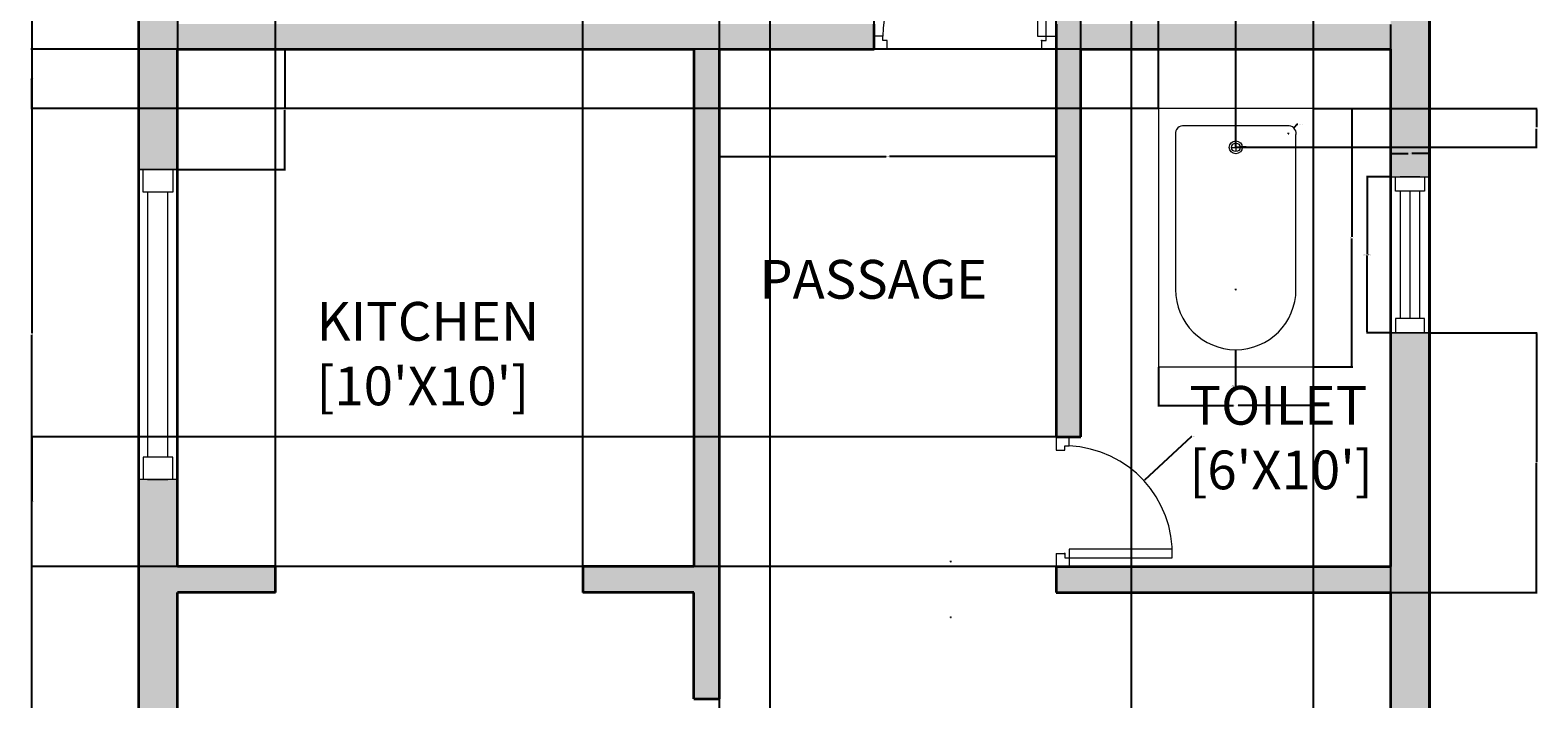
# Model space of a CAD drawing. Units: inches. Extents: x 2203 to 2554, y 381 to 929.
# Tile 2 of 3: x 2203 to 2554, y 570 to 726. Entities that reach past the tile are written whole.
import ezdxf

# ---------------------------------------------------------------- set-up
doc = ezdxf.new("R2010")
doc.units = ezdxf.units.IN
for name, color, linetype, lineweight in [('A-ANNO-DIMS', 2, 'Continuous', 18), ('A-AREA-IDEN', 7, 'Continuous', 18), ('A-DOOR', 239, 'Continuous', 18), ('A-FLOR-FIXT', 8, 'Continuous', 18), ('A-GLAZ', 4, 'Continuous', 18), ('A-WALL', 7, 'Continuous', 35), ('A-WALL-PATT', 250, 'Continuous', 13)]:
    doc.layers.add(name, color=color, linetype=linetype, lineweight=lineweight)
doc.styles.get("Standard").update_dxf_attribs({"font": 'arial.ttf'})
doc.dimstyles.get("Standard").update_dxf_attribs({"dimtxt": 0.18, "dimasz": 0.18, "dimexe": 0.18, "dimexo": 0.0625, "dimgap": 0.09, "dimtad": 0, "dimtih": 1, "dimtoh": 1, "dimdec": 4, "dimzin": 0, "dimdsep": 46, "dimtxsty": 'Standard', "dimcen": 0.09, "dimadec": 0, "dimazin": 0, "dimtfac": 1, "dimtdec": 4, "dimtofl": 0, "dimtmove": 0, "dimatfit": 3, "dimfxl": 1, "dimtolj": 1, "dimtzin": 0, "dimarcsym": 0})

# ---------------------------------------------------------------- blocks, each defined once
blk = doc.blocks.new('WIN-36')
for p, q in [((0, 36.19), (9, 36.19)), ((0, 0), (0, 36.19)), ((0, 36.19), (4.5, 36.19)), ((1.12, 32.87), (1.12, 36.19)), ((6.76, 36.19), (2.25, 36.19)), ((7.88, 36.19), (7.88, 32.87)), ((9, 36.19), (9, 0)), ((7.88, 32.87), (1.12, 32.87)), ((2.25, 32.87), (2.25, 3.32)), ((4.5, 32.87), (4.5, 3.32)), ((6.76, 3.32), (6.76, 32.87)), ((9, 0), (0, 0)), ((2.25, 0), (0, 0)), ((0, 0), (6.76, 0)), ((7.88, 3.32), (1.12, 3.32)), ((1.12, 3.32), (1.12, 0)), ((4.5, 0), (6.76, 0)), ((6.76, 0), (9, 0)), ((7.88, 0), (7.88, 3.32))]:
    blk.add_line(p, q)
blk = doc.blocks.new('WIN-72')
for p, q in [((0, 0), (0, 9)), ((0, 9), (72, 9)), ((5.2, 7.99), (0, 7.99)), ((5.2, 1.13), (5.2, 7.99)), ((66.8, 1.13), (66.8, 7.99)), ((66.8, 7.99), (72, 7.99)), ((72, 9), (72, 0)), ((72, 6.99), (72, 9)), ((0, 6.99), (0, 2.25)), ((0, 0), (0, 4.5)), ((66.8, 6.99), (5.2, 6.99)), ((72, 4.5), (72, 6.99)), ((72, 2.25), (72, 6.99)), ((0, 1.13), (5.2, 1.13)), ((72, 0), (0, 0)), ((5.2, 2.25), (66.8, 2.25)), ((72, 1.13), (66.8, 1.13)), ((72, 0), (72, 2.25))]:
    blk.add_line(p, q)
blk = doc.blocks.new('TUB-36X60')
for p, q in [((17, 51), (19, 51)), ((18, 52), (18, 50))]:
    blk.add_line(p, q)
blk.add_lwpolyline([(36, 60), (0, 60), (0, 0), (36, 0)], close=True)
for points in [[(4, 54), (4, 18)], [(30, 56), (6, 56)], [(32, 18), (32, 54)]]:
    blk.add_lwpolyline(points)
for radius in [1.5, 1]:
    blk.add_circle((18, 51), radius)
for centre, radius, start, end in [((5.75, 54.25), 1.77, 81.8699, 188.1301), ((30.25, 54.25), 1.77, 351.8699, 98.1301), ((18, 18), 14, 180, 0)]:
    blk.add_arc(centre, radius, start, end)
blk = doc.blocks.new('*D17')
at = {"layer": 'A-ANNO-DIMS', "color": 0, "lineweight": -2, "transparency": 16777216}
for p, q in [((2519.54, 691.56), (2513.99, 691.56)), ((2514.17, 691.38), (2514.17, 673.65)), ((2514.17, 655.55), (2514.17, 673.28)), ((2519.54, 655.37), (2513.99, 655.37))]:
    blk.add_line(p, q, dxfattribs=at)
at = {"layer": 'A-ANNO-DIMS', "color": 0, "transparency": 16777216}
for points in [[(2514.14, 691.38), (2514.2, 691.38), (2514.17, 691.56)], [(2514.14, 655.55), (2514.2, 655.55), (2514.17, 655.37)]]:
    blk.add_solid(points, dxfattribs=at)
at = {"layer": 'Defpoints', "color": 0, "transparency": 16777216}
for p in [(2514.17, 691.56), (2519.6, 691.56), (2519.6, 655.37)]:
    blk.add_point(p, dxfattribs=at)
at = {"layer": 'A-ANNO-DIMS', "color": 0, "transparency": 16777216, "insert": (2514.17, 673.46), "char_height": 0.18, "attachment_point": 5}
blk.add_mtext('\\A1;WINDOW 36 TYP.', dxfattribs=at)
blk = doc.blocks.new('*D18')
at = {"layer": 'A-ANNO-DIMS', "color": 0, "lineweight": -2, "transparency": 16777216}
for p, q in [((2519.6, 691.62), (2519.6, 697.17)), ((2519.78, 696.99), (2523.64, 696.99)), ((2528.42, 696.99), (2524.56, 696.99)), ((2528.6, 691.62), (2528.6, 697.17))]:
    blk.add_line(p, q, dxfattribs=at)
at = {"layer": 'A-ANNO-DIMS', "color": 0, "transparency": 16777216}
for points in [[(2519.78, 697.02), (2519.78, 696.96), (2519.6, 696.99)], [(2528.42, 697.02), (2528.42, 696.96), (2528.6, 696.99)]]:
    blk.add_solid(points, dxfattribs=at)
at = {"layer": 'Defpoints', "color": 0, "transparency": 16777216}
for p in [(2528.6, 696.99), (2519.6, 691.56), (2528.6, 691.56)]:
    blk.add_point(p, dxfattribs=at)
at = {"layer": 'A-ANNO-DIMS', "color": 0, "transparency": 16777216, "insert": (2524.1, 696.99), "char_height": 0.18, "attachment_point": 5}
blk.add_mtext('\\A1;9 TYP.', dxfattribs=at)
blk = doc.blocks.new('*D19')
at = {"layer": 'A-ANNO-DIMS', "color": 0, "lineweight": -2, "transparency": 16777216}
for p, q in [((2501.66, 707.44), (2510.78, 707.44)), ((2510.6, 707.26), (2510.6, 677.62)), ((2510.6, 647.62), (2510.6, 677.25)), ((2501.66, 647.44), (2510.78, 647.44))]:
    blk.add_line(p, q, dxfattribs=at)
at = {"layer": 'A-ANNO-DIMS', "color": 0, "transparency": 16777216}
for points in [[(2510.57, 707.26), (2510.63, 707.26), (2510.6, 707.44)], [(2510.57, 647.62), (2510.63, 647.62), (2510.6, 647.44)]]:
    blk.add_solid(points, dxfattribs=at)
at = {"layer": 'Defpoints', "color": 0, "transparency": 16777216}
for p in [(2501.6, 707.44), (2510.6, 707.44), (2501.6, 647.44)]:
    blk.add_point(p, dxfattribs=at)
at = {"layer": 'A-ANNO-DIMS', "color": 0, "transparency": 16777216, "insert": (2510.6, 677.44), "char_height": 0.18, "attachment_point": 5}
blk.add_mtext('\\A1;TUB 60 TYP.', dxfattribs=at)
blk = doc.blocks.new('*D20')
at = {"layer": 'A-ANNO-DIMS', "color": 0, "lineweight": -2, "transparency": 16777216}
for p, q in [((2465.6, 647.37), (2465.6, 638.26)), ((2501.6, 647.37), (2501.6, 638.26)), ((2465.78, 638.44), (2483.07, 638.44)), ((2501.42, 638.44), (2484.13, 638.44))]:
    blk.add_line(p, q, dxfattribs=at)
at = {"layer": 'A-ANNO-DIMS', "color": 0, "transparency": 16777216}
for points in [[(2465.78, 638.47), (2465.78, 638.41), (2465.6, 638.44)], [(2501.42, 638.47), (2501.42, 638.41), (2501.6, 638.44)]]:
    blk.add_solid(points, dxfattribs=at)
at = {"layer": 'Defpoints', "color": 0, "transparency": 16777216}
for p in [(2465.6, 647.44), (2501.6, 647.44), (2501.6, 638.44)]:
    blk.add_point(p, dxfattribs=at)
at = {"layer": 'A-ANNO-DIMS', "color": 0, "transparency": 16777216, "insert": (2483.6, 638.44), "char_height": 0.18, "attachment_point": 5}
blk.add_mtext('\\A1;36 TYP.', dxfattribs=at)
blk = doc.blocks.new('*D22')
at = {"layer": 'A-ANNO-DIMS', "color": 0, "lineweight": -2, "transparency": 16777216}
for p, q in [((2228.54, 904.06), (2203.5, 904.06)), ((2203.68, 903.88), (2203.68, 655.25)), ((2203.68, 406.24), (2203.68, 654.88)), ((2228.54, 406.06), (2203.5, 406.06))]:
    blk.add_line(p, q, dxfattribs=at)
at = {"layer": 'A-ANNO-DIMS', "color": 0, "transparency": 16777216}
for points in [[(2203.65, 903.88), (2203.71, 903.88), (2203.68, 904.06)], [(2203.65, 406.24), (2203.71, 406.24), (2203.68, 406.06)]]:
    blk.add_solid(points, dxfattribs=at)
at = {"layer": 'Defpoints', "color": 0, "transparency": 16777216}
for p in [(2203.68, 904.06), (2228.6, 904.06), (2228.6, 406.06)]:
    blk.add_point(p, dxfattribs=at)
at = {"layer": 'A-ANNO-DIMS', "color": 0, "transparency": 16777216, "insert": (2203.68, 655.06), "char_height": 0.18, "attachment_point": 5}
blk.add_mtext('\\A1;498', dxfattribs=at)
blk = doc.blocks.new('*D26')
at = {"layer": 'A-ANNO-DIMS', "color": 0, "lineweight": -2, "transparency": 16777216}
for p, q in [((2237.66, 721.24), (2262.7, 721.24)), ((2262.52, 721.06), (2262.52, 707.43)), ((2262.52, 693.44), (2262.52, 707.07)), ((2237.66, 693.26), (2262.7, 693.26))]:
    blk.add_line(p, q, dxfattribs=at)
at = {"layer": 'A-ANNO-DIMS', "color": 0, "transparency": 16777216}
for points in [[(2262.49, 721.06), (2262.55, 721.06), (2262.52, 721.24)], [(2262.49, 693.44), (2262.55, 693.44), (2262.52, 693.26)]]:
    blk.add_solid(points, dxfattribs=at)
at = {"layer": 'Defpoints', "color": 0, "transparency": 16777216}
for p in [(2237.6, 721.24), (2237.6, 693.26), (2262.52, 693.26)]:
    blk.add_point(p, dxfattribs=at)
at = {"layer": 'A-ANNO-DIMS', "color": 0, "transparency": 16777216, "insert": (2262.52, 707.25), "char_height": 0.18, "attachment_point": 5}
blk.add_mtext('\\A1;27.985', dxfattribs=at)
blk = doc.blocks.new('*D27')
at = {"layer": 'A-ANNO-DIMS', "color": 0, "lineweight": -2, "transparency": 16777216}
for p, q in [((2528.66, 655.37), (2553.7, 655.37)), ((2553.52, 655.19), (2553.52, 625.4)), ((2553.52, 595.24), (2553.52, 625.04)), ((2519.66, 595.06), (2553.7, 595.06))]:
    blk.add_line(p, q, dxfattribs=at)
at = {"layer": 'A-ANNO-DIMS', "color": 0, "transparency": 16777216}
for points in [[(2553.49, 655.19), (2553.55, 655.19), (2553.52, 655.37)], [(2553.49, 595.24), (2553.55, 595.24), (2553.52, 595.06)]]:
    blk.add_solid(points, dxfattribs=at)
at = {"layer": 'Defpoints', "color": 0, "transparency": 16777216}
for p in [(2528.6, 655.37), (2553.52, 655.37), (2519.6, 595.06)]:
    blk.add_point(p, dxfattribs=at)
at = {"layer": 'A-ANNO-DIMS', "color": 0, "transparency": 16777216, "insert": (2553.52, 625.22), "char_height": 0.18, "attachment_point": 5}
blk.add_mtext('\\A1;60.31', dxfattribs=at)
blk = doc.blocks.new('*D29')
at = {"layer": 'A-ANNO-DIMS', "color": 0, "lineweight": -2, "transparency": 16777216}
for p, q in [((2363.6, 721.18), (2363.6, 696.14)), ((2441.82, 721.18), (2441.82, 696.14)), ((2363.78, 696.32), (2402.32, 696.32)), ((2441.64, 696.32), (2403.1, 696.32))]:
    blk.add_line(p, q, dxfattribs=at)
at = {"layer": 'A-ANNO-DIMS', "color": 0, "transparency": 16777216}
for points in [[(2363.78, 696.35), (2363.78, 696.29), (2363.6, 696.32)], [(2441.64, 696.35), (2441.64, 696.29), (2441.82, 696.32)]]:
    blk.add_solid(points, dxfattribs=at)
at = {"layer": 'Defpoints', "color": 0, "transparency": 16777216}
for p in [(2363.6, 721.24), (2441.82, 721.24), (2363.6, 696.32)]:
    blk.add_point(p, dxfattribs=at)
at = {"layer": 'A-ANNO-DIMS', "color": 0, "transparency": 16777216, "insert": (2402.71, 696.32), "char_height": 0.18, "attachment_point": 5}
blk.add_mtext('\\A1;78.23', dxfattribs=at)
blk = doc.blocks.new('*D30')
at = {"layer": 'A-ANNO-DIMS', "color": 0, "lineweight": -2, "transparency": 16777216}
for p, q in [((2237.6, 601.13), (2237.6, 929.16)), ((2237.78, 928.98), (2248.57, 928.98)), ((2260.15, 928.98), (2249.36, 928.98)), ((2260.33, 601.13), (2260.33, 929.16))]:
    blk.add_line(p, q, dxfattribs=at)
at = {"layer": 'A-ANNO-DIMS', "color": 0, "transparency": 16777216}
for points in [[(2237.78, 929.01), (2237.78, 928.95), (2237.6, 928.98)], [(2260.15, 929.01), (2260.15, 928.95), (2260.33, 928.98)]]:
    blk.add_solid(points, dxfattribs=at)
at = {"layer": 'Defpoints', "color": 0, "transparency": 16777216}
for p in [(2260.33, 928.98), (2237.6, 601.06), (2260.33, 601.06)]:
    blk.add_point(p, dxfattribs=at)
at = {"layer": 'A-ANNO-DIMS', "color": 0, "transparency": 16777216, "insert": (2248.96, 928.98), "char_height": 0.18, "attachment_point": 5}
blk.add_mtext('\\A1;22.73', dxfattribs=at)
blk = doc.blocks.new('*D31')
at = {"layer": 'A-ANNO-DIMS', "color": 0, "lineweight": -2, "transparency": 16777216}
for p, q in [((2260.33, 601.13), (2260.33, 929.16)), ((2260.51, 928.98), (2295.75, 928.98)), ((2331.64, 928.98), (2296.4, 928.98)), ((2331.82, 601.13), (2331.82, 929.16))]:
    blk.add_line(p, q, dxfattribs=at)
at = {"layer": 'A-ANNO-DIMS', "color": 0, "transparency": 16777216}
for points in [[(2260.51, 929.01), (2260.51, 928.95), (2260.33, 928.98)], [(2331.64, 929.01), (2331.64, 928.95), (2331.82, 928.98)]]:
    blk.add_solid(points, dxfattribs=at)
at = {"layer": 'Defpoints', "color": 0, "transparency": 16777216}
for p in [(2331.82, 928.98), (2260.33, 601.06), (2331.82, 601.06)]:
    blk.add_point(p, dxfattribs=at)
at = {"layer": 'A-ANNO-DIMS', "color": 0, "transparency": 16777216, "insert": (2296.08, 928.98), "char_height": 0.18, "attachment_point": 5}
blk.add_mtext('\\A1;71.5', dxfattribs=at)
blk = doc.blocks.new('*D35')
at = {"layer": 'A-ANNO-DIMS', "color": 0, "lineweight": -2, "transparency": 16777216}
for p, q in [((2399.53, 721.31), (2399.53, 746.34)), ((2399.71, 746.16), (2420.28, 746.16)), ((2441.64, 746.16), (2421.08, 746.16)), ((2441.82, 721.31), (2441.82, 746.34))]:
    blk.add_line(p, q, dxfattribs=at)
at = {"layer": 'A-ANNO-DIMS', "color": 0, "transparency": 16777216}
for points in [[(2399.71, 746.19), (2399.71, 746.13), (2399.53, 746.16)], [(2441.64, 746.19), (2441.64, 746.13), (2441.82, 746.16)]]:
    blk.add_solid(points, dxfattribs=at)
at = {"layer": 'Defpoints', "color": 0, "transparency": 16777216}
for p in [(2441.82, 746.16), (2399.53, 721.24), (2441.82, 721.24)]:
    blk.add_point(p, dxfattribs=at)
at = {"layer": 'A-ANNO-DIMS', "color": 0, "transparency": 16777216, "insert": (2420.68, 746.16), "char_height": 0.18, "attachment_point": 5}
blk.add_mtext('\\A1;42.29', dxfattribs=at)
blk = doc.blocks.new('*D37')
at = {"layer": 'A-ANNO-DIMS', "color": 0, "lineweight": -2, "transparency": 16777216}
for p, q in [((2441.76, 631.17), (2203.5, 631.17)), ((2203.68, 630.99), (2203.68, 616.3)), ((2203.68, 601.24), (2203.68, 615.93)), ((2441.76, 601.06), (2203.5, 601.06))]:
    blk.add_line(p, q, dxfattribs=at)
at = {"layer": 'A-ANNO-DIMS', "color": 0, "transparency": 16777216}
for points in [[(2203.65, 630.99), (2203.71, 630.99), (2203.68, 631.17)], [(2203.65, 601.24), (2203.71, 601.24), (2203.68, 601.06)]]:
    blk.add_solid(points, dxfattribs=at)
at = {"layer": 'Defpoints', "color": 0, "transparency": 16777216}
for p in [(2203.68, 631.17), (2441.82, 631.17), (2441.82, 601.06)]:
    blk.add_point(p, dxfattribs=at)
at = {"layer": 'A-ANNO-DIMS', "color": 0, "transparency": 16777216, "insert": (2203.68, 616.12), "char_height": 0.18, "attachment_point": 5}
blk.add_mtext('\\A1;30.104', dxfattribs=at)
blk = doc.blocks.new('*D41')
at = {"layer": 'A-ANNO-DIMS', "color": 0, "lineweight": -2, "transparency": 16777216}
for p, q in [((2375.37, 509.13), (2375.37, 929.16)), ((2375.55, 928.98), (2417.15, 928.98)), ((2459.19, 928.98), (2417.59, 928.98)), ((2459.37, 509.13), (2459.37, 929.16))]:
    blk.add_line(p, q, dxfattribs=at)
at = {"layer": 'A-ANNO-DIMS', "color": 0, "transparency": 16777216}
for points in [[(2375.55, 929.01), (2375.55, 928.95), (2375.37, 928.98)], [(2459.19, 929.01), (2459.19, 928.95), (2459.37, 928.98)]]:
    blk.add_solid(points, dxfattribs=at)
at = {"layer": 'Defpoints', "color": 0, "transparency": 16777216}
for p in [(2459.37, 928.98), (2375.37, 509.06), (2459.37, 509.06)]:
    blk.add_point(p, dxfattribs=at)
at = {"layer": 'A-ANNO-DIMS', "color": 0, "transparency": 16777216, "insert": (2417.37, 928.98), "char_height": 0.18, "attachment_point": 5}
blk.add_mtext('\\A1;84', dxfattribs=at)
blk = doc.blocks.new('*D43')
at = {"layer": 'A-ANNO-DIMS', "color": 0, "lineweight": -2, "transparency": 16777216}
for p, q in [((2363.6, 500.21), (2363.6, 929.16)), ((2363.78, 928.98), (2369.03, 928.98)), ((2375.19, 928.98), (2369.94, 928.98)), ((2375.37, 509.13), (2375.37, 929.16))]:
    blk.add_line(p, q, dxfattribs=at)
at = {"layer": 'A-ANNO-DIMS', "color": 0, "transparency": 16777216}
for points in [[(2363.78, 929.01), (2363.78, 928.95), (2363.6, 928.98)], [(2375.19, 929.01), (2375.19, 928.95), (2375.37, 928.98)]]:
    blk.add_solid(points, dxfattribs=at)
at = {"layer": 'Defpoints', "color": 0, "transparency": 16777216}
for p in [(2375.37, 928.98), (2375.37, 509.06), (2363.6, 500.15)]:
    blk.add_point(p, dxfattribs=at)
at = {"layer": 'A-ANNO-DIMS', "color": 0, "transparency": 16777216, "insert": (2369.49, 928.98), "char_height": 0.18, "attachment_point": 5}
blk.add_mtext('\\A1;11.775', dxfattribs=at)
blk = doc.blocks.new('*D50')
at = {"layer": 'A-ANNO-DIMS', "color": 0, "lineweight": -2, "transparency": 16777216}
for p, q in [((2465.6, 707.5), (2465.6, 929.16)), ((2465.78, 928.98), (2474.39, 928.98)), ((2483.42, 928.98), (2474.81, 928.98)), ((2483.6, 698.5), (2483.6, 929.16))]:
    blk.add_line(p, q, dxfattribs=at)
at = {"layer": 'A-ANNO-DIMS', "color": 0, "transparency": 16777216}
for points in [[(2465.78, 929.01), (2465.78, 928.95), (2465.6, 928.98)], [(2483.42, 929.01), (2483.42, 928.95), (2483.6, 928.98)]]:
    blk.add_solid(points, dxfattribs=at)
at = {"layer": 'Defpoints', "color": 0, "transparency": 16777216}
for p in [(2483.6, 928.98), (2465.6, 707.44), (2483.6, 698.44)]:
    blk.add_point(p, dxfattribs=at)
at = {"layer": 'A-ANNO-DIMS', "color": 0, "transparency": 16777216, "insert": (2474.6, 928.98), "char_height": 0.18, "attachment_point": 5}
blk.add_mtext('\\A1;18', dxfattribs=at)
blk = doc.blocks.new('*D51')
at = {"layer": 'A-ANNO-DIMS', "color": 0, "lineweight": -2, "transparency": 16777216}
for p, q in [((2501.66, 707.44), (2553.7, 707.44)), ((2553.52, 707.26), (2553.52, 703.12)), ((2553.52, 698.62), (2553.52, 702.75)), ((2483.66, 698.44), (2553.7, 698.44))]:
    blk.add_line(p, q, dxfattribs=at)
at = {"layer": 'A-ANNO-DIMS', "color": 0, "transparency": 16777216}
for points in [[(2553.49, 707.26), (2553.55, 707.26), (2553.52, 707.44)], [(2553.49, 698.62), (2553.55, 698.62), (2553.52, 698.44)]]:
    blk.add_solid(points, dxfattribs=at)
at = {"layer": 'Defpoints', "color": 0, "transparency": 16777216}
for p in [(2501.6, 707.44), (2483.6, 698.44), (2553.52, 698.44)]:
    blk.add_point(p, dxfattribs=at)
at = {"layer": 'A-ANNO-DIMS', "color": 0, "transparency": 16777216, "insert": (2553.52, 702.94), "char_height": 0.18, "attachment_point": 5}
blk.add_mtext('\\A1;9', dxfattribs=at)
blk = doc.blocks.new('*D52')
at = {"layer": 'A-ANNO-DIMS', "color": 0, "lineweight": -2, "transparency": 16777216}
for p, q in [((2447.6, 721.31), (2447.6, 929.16)), ((2447.78, 928.98), (2456.39, 928.98)), ((2465.42, 928.98), (2456.81, 928.98)), ((2465.6, 707.5), (2465.6, 929.16))]:
    blk.add_line(p, q, dxfattribs=at)
at = {"layer": 'A-ANNO-DIMS', "color": 0, "transparency": 16777216}
for points in [[(2447.78, 929.01), (2447.78, 928.95), (2447.6, 928.98)], [(2465.42, 929.01), (2465.42, 928.95), (2465.6, 928.98)]]:
    blk.add_solid(points, dxfattribs=at)
at = {"layer": 'Defpoints', "color": 0, "transparency": 16777216}
for p in [(2447.6, 928.98), (2447.6, 721.24), (2465.6, 707.44)]:
    blk.add_point(p, dxfattribs=at)
at = {"layer": 'A-ANNO-DIMS', "color": 0, "transparency": 16777216, "insert": (2456.6, 928.98), "char_height": 0.18, "attachment_point": 5}
blk.add_mtext('\\A1;18', dxfattribs=at)
blk = doc.blocks.new('*D53')
at = {"layer": 'A-ANNO-DIMS', "color": 0, "lineweight": -2, "transparency": 16777216}
for p, q in [((2447.54, 721.24), (2203.5, 721.24)), ((2203.68, 721.06), (2203.68, 714.52)), ((2203.68, 707.62), (2203.68, 714.16)), ((2465.54, 707.44), (2203.5, 707.44))]:
    blk.add_line(p, q, dxfattribs=at)
at = {"layer": 'A-ANNO-DIMS', "color": 0, "transparency": 16777216}
for points in [[(2203.65, 721.06), (2203.71, 721.06), (2203.68, 721.24)], [(2203.65, 707.62), (2203.71, 707.62), (2203.68, 707.44)]]:
    blk.add_solid(points, dxfattribs=at)
at = {"layer": 'Defpoints', "color": 0, "transparency": 16777216}
for p in [(2203.68, 721.24), (2447.6, 721.24), (2465.6, 707.44)]:
    blk.add_point(p, dxfattribs=at)
at = {"layer": 'A-ANNO-DIMS', "color": 0, "transparency": 16777216, "insert": (2203.68, 714.34), "char_height": 0.18, "attachment_point": 5}
blk.add_mtext('\\A1;13.808', dxfattribs=at)
blk = doc.blocks.new('*D55')
at = {"layer": 'A-ANNO-DIMS', "color": 0, "lineweight": -2, "transparency": 16777216}
for p, q in [((2501.6, 739.61), (2501.6, 380.96)), ((2519.6, 727), (2519.6, 380.96)), ((2501.78, 381.14), (2510.39, 381.14)), ((2519.42, 381.14), (2510.81, 381.14))]:
    blk.add_line(p, q, dxfattribs=at)
at = {"layer": 'A-ANNO-DIMS', "color": 0, "transparency": 16777216}
for points in [[(2501.78, 381.17), (2501.78, 381.11), (2501.6, 381.14)], [(2519.42, 381.17), (2519.42, 381.11), (2519.6, 381.14)]]:
    blk.add_solid(points, dxfattribs=at)
at = {"layer": 'Defpoints', "color": 0, "transparency": 16777216}
for p in [(2501.6, 739.68), (2519.6, 727.06), (2519.6, 381.14)]:
    blk.add_point(p, dxfattribs=at)
at = {"layer": 'A-ANNO-DIMS', "color": 0, "transparency": 16777216, "insert": (2510.6, 381.14), "char_height": 0.18, "attachment_point": 5}
blk.add_mtext('\\A1;18', dxfattribs=at)
blk = doc.blocks.new('*D60')
at = {"layer": 'A-ANNO-DIMS', "color": 0, "lineweight": -2, "transparency": 16777216}
for p, q in [((2417.28, 602.26), (2417.46, 602.26)), ((2417.37, 602.17), (2417.37, 602.35)), ((2417.37, 408.35), (2417.37, 480.88)), ((2417.55, 408.35), (2417.37, 408.35))]:
    blk.add_line(p, q, dxfattribs=at)
at = {"layer": 'A-ANNO-DIMS', "color": 0, "transparency": 16777216}
blk.add_solid([(2417.4, 480.88), (2417.34, 480.88), (2417.37, 481.06)], dxfattribs=at)
at = {"layer": 'Defpoints', "color": 0, "transparency": 16777216}
for p in [(2417.37, 602.26), (2417.37, 481.06)]:
    blk.add_point(p, dxfattribs=at)
at = {"layer": 'A-ANNO-DIMS', "color": 0, "transparency": 16777216, "insert": (2418.03, 408.35), "char_height": 0.18, "attachment_point": 5}
blk.add_mtext('\\A1;R121.2', dxfattribs=at)
blk = doc.blocks.new('*D61')
at = {"layer": 'A-ANNO-DIMS', "color": 0, "lineweight": -2, "transparency": 16777216}
for p, q in [((2417.28, 589.31), (2417.46, 589.31)), ((2417.37, 589.22), (2417.37, 589.4)), ((2417.37, 406.51), (2417.37, 474.88)), ((2417.55, 406.51), (2417.37, 406.51))]:
    blk.add_line(p, q, dxfattribs=at)
at = {"layer": 'A-ANNO-DIMS', "color": 0, "transparency": 16777216}
blk.add_solid([(2417.4, 474.88), (2417.34, 474.88), (2417.37, 475.06)], dxfattribs=at)
at = {"layer": 'Defpoints', "color": 0, "transparency": 16777216}
for p in [(2417.37, 589.31), (2417.37, 475.06)]:
    blk.add_point(p, dxfattribs=at)
at = {"layer": 'A-ANNO-DIMS', "color": 0, "transparency": 16777216, "insert": (2418.1, 406.51), "char_height": 0.18, "attachment_point": 5}
blk.add_mtext('\\A1;R114.25', dxfattribs=at)
blk = doc.blocks.new('*D63')
at = {"layer": 'A-ANNO-DIMS', "color": 0, "lineweight": -2, "transparency": 16777216}
for p, q in [((2397.62, 766.24), (2397.8, 766.24)), ((2397.8, 766.24), (2412.95, 750.24)), ((2438.44, 723.24), (2438.62, 723.24)), ((2438.53, 723.15), (2438.53, 723.33))]:
    blk.add_line(p, q, dxfattribs=at)
at = {"layer": 'A-ANNO-DIMS', "color": 0, "transparency": 16777216}
blk.add_solid([(2412.97, 750.27), (2412.93, 750.22), (2413.08, 750.11)], dxfattribs=at)
at = {"layer": 'Defpoints', "color": 0, "transparency": 16777216}
for p in [(2413.08, 750.11), (2438.53, 723.24)]:
    blk.add_point(p, dxfattribs=at)
at = {"layer": 'A-ANNO-DIMS', "color": 0, "transparency": 16777216, "insert": (2397.16, 766.24), "char_height": 0.18, "attachment_point": 5}
blk.add_mtext('\\A1;R37.01', dxfattribs=at)
blk = doc.blocks.new('*D65')
at = {"layer": 'A-ANNO-DIMS', "color": 0, "lineweight": -2, "transparency": 16777216}
for p, q in [((2473.24, 631.22), (2462.34, 621.16)), ((2473.42, 631.22), (2473.24, 631.22)), ((2443.73, 604.06), (2443.91, 604.06)), ((2443.82, 603.97), (2443.82, 604.15))]:
    blk.add_line(p, q, dxfattribs=at)
at = {"layer": 'A-ANNO-DIMS', "color": 0, "transparency": 16777216}
blk.add_solid([(2462.32, 621.18), (2462.36, 621.14), (2462.21, 621.04)], dxfattribs=at)
at = {"layer": 'Defpoints', "color": 0, "transparency": 16777216}
for p in [(2462.21, 621.04), (2443.82, 604.06)]:
    blk.add_point(p, dxfattribs=at)
at = {"layer": 'A-ANNO-DIMS', "color": 0, "transparency": 16777216, "insert": (2473.9, 631.22), "char_height": 0.18, "attachment_point": 5}
blk.add_mtext('\\A1;R25.02', dxfattribs=at)
blk = doc.blocks.new('*D66')
at = {"layer": 'A-ANNO-DIMS', "color": 0, "lineweight": -2, "transparency": 16777216}
for p, q in [((2483.51, 665.44), (2483.69, 665.44)), ((2483.6, 665.35), (2483.6, 665.53)), ((2483.6, 643.04), (2483.6, 651.26)), ((2483.42, 643.04), (2483.6, 643.04))]:
    blk.add_line(p, q, dxfattribs=at)
at = {"layer": 'A-ANNO-DIMS', "color": 0, "transparency": 16777216}
blk.add_solid([(2483.57, 651.26), (2483.63, 651.26), (2483.6, 651.44)], dxfattribs=at)
at = {"layer": 'Defpoints', "color": 0, "transparency": 16777216}
for p in [(2483.6, 665.44), (2483.6, 651.44)]:
    blk.add_point(p, dxfattribs=at)
at = {"layer": 'A-ANNO-DIMS', "color": 0, "transparency": 16777216, "insert": (2482.92, 643.04), "char_height": 0.18, "attachment_point": 5}
blk.add_mtext('\\A1;2X R14', dxfattribs=at)
blk = doc.blocks.new('*D67')
at = {"layer": 'A-ANNO-DIMS', "color": 0, "lineweight": -2, "transparency": 16777216}
for p, q in [((2483.51, 698.44), (2483.69, 698.44)), ((2483.6, 698.35), (2483.6, 698.53)), ((2485.2, 698.44), (2484.78, 698.44))]:
    blk.add_line(p, q, dxfattribs=at)
at = {"layer": 'A-ANNO-DIMS', "color": 0, "transparency": 16777216}
blk.add_solid([(2484.78, 698.47), (2484.78, 698.41), (2484.6, 698.44)], dxfattribs=at)
at = {"layer": 'Defpoints', "color": 0, "transparency": 16777216}
for p in [(2482.6, 698.43), (2484.6, 698.44)]:
    blk.add_point(p, dxfattribs=at)
at = {"layer": 'A-ANNO-DIMS', "color": 0, "transparency": 16777216, "insert": (2485.64, 698.44), "char_height": 0.18, "attachment_point": 5}
blk.add_mtext('\\A1;2X ∅2', dxfattribs=at)
blk = doc.blocks.new('*D68')
at = {"layer": 'A-ANNO-DIMS', "color": 0, "lineweight": -2, "transparency": 16777216}
for p, q in [((2483.51, 698.44), (2483.69, 698.44)), ((2483.6, 698.35), (2483.6, 698.53)), ((2486, 698.44), (2485.28, 698.44))]:
    blk.add_line(p, q, dxfattribs=at)
at = {"layer": 'A-ANNO-DIMS', "color": 0, "transparency": 16777216}
blk.add_solid([(2485.28, 698.47), (2485.28, 698.41), (2485.1, 698.44)], dxfattribs=at)
at = {"layer": 'Defpoints', "color": 0, "transparency": 16777216}
for p in [(2482.1, 698.43), (2485.1, 698.44)]:
    blk.add_point(p, dxfattribs=at)
at = {"layer": 'A-ANNO-DIMS', "color": 0, "transparency": 16777216, "insert": (2486.44, 698.44), "char_height": 0.18, "attachment_point": 5}
blk.add_mtext('\\A1;2X ∅3', dxfattribs=at)
blk = doc.blocks.new('*D69')
at = {"layer": 'A-ANNO-DIMS', "color": 0, "lineweight": -2, "transparency": 16777216}
for p, q in [((2495.76, 701.69), (2495.94, 701.69)), ((2495.85, 701.6), (2495.85, 701.78)), ((2497.83, 703.71), (2497.21, 703.08)), ((2498.01, 703.71), (2497.83, 703.71))]:
    blk.add_line(p, q, dxfattribs=at)
at = {"layer": 'A-ANNO-DIMS', "color": 0, "transparency": 16777216}
blk.add_solid([(2497.19, 703.1), (2497.23, 703.06), (2497.09, 702.95)], dxfattribs=at)
at = {"layer": 'Defpoints', "color": 0, "transparency": 16777216}
for p in [(2495.85, 701.69), (2497.09, 702.95)]:
    blk.add_point(p, dxfattribs=at)
at = {"layer": 'A-ANNO-DIMS', "color": 0, "transparency": 16777216, "insert": (2498.62, 703.71), "char_height": 0.18, "attachment_point": 5}
blk.add_mtext('\\A1;4X R1.77', dxfattribs=at)

msp = doc.modelspace()

# ---------------------------------------------------------------- hatches: boundary and pattern name
at = {"layer": 'A-WALL-PATT'}
h = msp.add_hatch(color=256, dxfattribs=at)
h.dxf.hatch_style = 1
h.paths.add_polyline_path([(2237.599, 595.0647), (2260.3281, 595.0647), (2260.3281, 601.0647), (2237.599, 601.0647), (2237.599, 621.2584), (2233.099, 621.2584), (2230.6109, 621.2584), (2228.599, 621.2584), (2228.599, 466.0647), (2261.0302, 466.0647), (2261.0302, 470.5647), (2261.0302, 473.0528), (2261.0302, 475.0647), (2237.599, 475.0647)])
h.paths.add_polyline_path([(2237.599, 895.0647), (2305.0273, 895.0647), (2305.0273, 899.5647), (2305.0273, 904.0647), (2228.599, 904.0647), (2228.599, 693.2584), (2230.6109, 693.2584), (2235.349, 693.2584), (2237.599, 693.2584), (2237.599, 721.2436), (2357.599, 721.2436), (2357.599, 601.0647), (2331.8237, 601.0647), (2331.8237, 595.0647), (2357.599, 595.0647), (2357.599, 570.3283), (2363.599, 570.3283), (2363.599, 595.0647), (2363.599, 601.0647), (2363.599, 721.2436), (2399.5308, 721.2436), (2399.5308, 724.2436), (2399.5308, 727.0647), (2237.599, 727.0647)])
h.paths.add_polyline_path([(2447.599, 859.3877), (2441.8244, 859.3877), (2441.8244, 727.0647), (2441.8244, 721.2436), (2441.8244, 691.5632), (2441.8244, 631.1686), (2444.8244, 631.1686), (2447.599, 631.1686), (2447.599, 721.2436), (2519.599, 721.2436), (2519.599, 691.5572), (2524.099, 691.5572), (2526.3564, 691.5572), (2528.599, 691.5572), (2528.599, 904.0647), (2496.9662, 904.0647), (2496.9662, 901.8221), (2496.9662, 895.0647), (2519.599, 895.0647), (2519.599, 727.0647), (2447.599, 727.0647)])
h.paths.add_polyline_path([(2460.78, 904.0647), (2377.0273, 904.0647), (2377.0273, 902.0528), (2377.0273, 895.0647), (2441.8244, 895.0647), (2460.78, 895.0647), (2460.78, 899.5647)])
h.paths.add_polyline_path([(2471.599, 475.0647), (2363.599, 475.0647), (2363.599, 500.1465), (2357.599, 500.1465), (2357.599, 475.0647), (2333.0302, 475.0647), (2333.0302, 473.0528), (2333.0302, 468.3147), (2333.0302, 466.0647), (2471.599, 466.0647), (2471.599, 469.0647)])
h = msp.add_hatch(color=256, dxfattribs=at)
h.dxf.hatch_style = 1
h.paths.add_polyline_path([(2528.599, 655.371), (2526.3564, 655.371), (2519.599, 655.371), (2519.599, 601.0647), (2441.8244, 601.0647), (2441.8244, 595.0647), (2519.599, 595.0647), (2519.599, 475.0647), (2519.599, 466.0647), (2528.599, 466.0647)])

# ---------------------------------------------------------------- linework, layer by layer
at = {"layer": 'A-DOOR'}
for p, q in [((2437.5308, 760.2436), (2437.5308, 724.2436)), ((2439.5308, 724.2436), (2439.5308, 760.2436)), ((2399.5308, 724.2436), (2399.5308, 721.2436)), ((2401.5308, 724.2436), (2399.5308, 724.2436)), ((2401.5308, 723.2436), (2401.5308, 724.2436)), ((2402.5308, 723.2436), (2401.5308, 723.2436)), ((2402.5308, 721.2436), (2402.5308, 723.2436)), ((2437.5308, 724.2436), (2439.5308, 724.2436)), ((2438.5308, 721.2436), (2438.5308, 723.2436)), ((2438.5308, 723.2436), (2439.5308, 723.2436)), ((2439.5308, 723.2436), (2439.5308, 724.2436)), ((2439.5308, 724.2436), (2441.8244, 724.2436)), ((2441.8244, 724.2436), (2441.8244, 721.2436)), ((2399.5308, 721.2436), (2402.5308, 721.2436)), ((2399.5308, 721.2436), (2402.5308, 721.2436)), ((2438.5308, 721.2436), (2441.8244, 721.2436)), ((2444.8244, 631.1686), (2441.8244, 631.1686)), ((2441.8244, 631.1686), (2441.8244, 628.0647)), ((2441.8244, 631.1686), (2441.8244, 628.0647)), ((2444.8244, 629.0647), (2444.8244, 631.1686)), ((2441.8244, 628.0647), (2443.8244, 628.0647)), ((2443.8244, 628.0647), (2443.8244, 629.0647)), ((2443.8244, 629.0647), (2444.8244, 629.0647)), ((2441.8244, 604.0647), (2443.8244, 604.0647)), ((2441.8244, 604.0647), (2441.8244, 601.0647)), ((2443.8244, 604.0647), (2443.8244, 603.0647)), ((2443.8244, 603.0647), (2444.8244, 603.0647)), ((2468.8244, 605.0647), (2444.8244, 605.0647)), ((2444.8244, 605.0647), (2444.8244, 603.0647)), ((2444.8244, 603.0647), (2444.8244, 601.0647)), ((2444.8244, 603.0647), (2468.8244, 603.0647)), ((2468.8244, 603.0647), (2468.8244, 605.0647)), ((2444.8244, 601.0647), (2441.8244, 601.0647))]:
    msp.add_line(p, q, dxfattribs=at)
for centre, radius, start, end in [((2438.5308, 723.2436), 37.0135, 88.451842, 178.451842), ((2443.8244, 604.0647), 25.02, 357.70939, 87.70939)]:
    msp.add_arc(centre, radius, start, end, dxfattribs=at)
at = {"layer": 'A-WALL'}
for p, q in [((2228.599, 466.0647), (2228.599, 904.0647)), ((2528.599, 904.0647), (2528.599, 466.0647)), ((2528.599, 466.0647), (2528.599, 904.0647)), ((2399.5308, 721.2436), (2399.5308, 727.0647)), ((2441.8244, 727.0647), (2441.8244, 721.2436)), ((2237.599, 601.0647), (2237.599, 721.2436)), ((2237.599, 721.2436), (2357.599, 721.2436)), ((2237.599, 601.0647), (2237.599, 721.2436)), ((2357.599, 721.2436), (2357.599, 601.0647)), ((2363.599, 601.0647), (2363.599, 721.2436)), ((2363.599, 721.2436), (2399.5308, 721.2436)), ((2441.8244, 721.2436), (2441.8244, 631.1686)), ((2441.8244, 721.2436), (2441.8244, 691.5632)), ((2447.599, 721.2436), (2519.599, 721.2436)), ((2447.599, 631.1686), (2447.599, 721.2436)), ((2519.599, 721.2436), (2519.599, 601.0647)), ((2441.8244, 631.1686), (2447.599, 631.1686)), ((2260.3281, 601.0647), (2237.599, 601.0647)), ((2260.3281, 595.0647), (2260.3281, 601.0647)), ((2357.599, 601.0647), (2331.8237, 601.0647)), ((2331.8237, 601.0647), (2331.8237, 595.0647)), ((2363.599, 595.0647), (2363.599, 601.0647)), ((2441.8244, 601.0647), (2519.599, 601.0647)), ((2441.8244, 601.0647), (2447.599, 601.0647)), ((2441.8244, 601.0647), (2441.8244, 595.0647)), ((2237.599, 475.0647), (2237.599, 595.0647)), ((2260.3281, 595.0647), (2237.599, 595.0647)), ((2357.599, 595.0647), (2331.8237, 595.0647)), ((2357.599, 570.3283), (2357.599, 595.0647)), ((2363.599, 570.3283), (2363.599, 595.0647)), ((2441.8244, 595.0647), (2519.599, 595.0647)), ((2519.599, 595.0647), (2519.599, 475.0647)), ((2357.599, 570.3283), (2363.599, 570.3283))]:
    msp.add_line(p, q, dxfattribs=at)

# ---------------------------------------------------------------- block references
at = {"layer": 'A-FLOR-FIXT'}
msp.add_blockref('TUB-36X60', (2465.599, 647.4353), dxfattribs=at)
at = {"layer": 'A-GLAZ', "rotation": 90}
msp.add_blockref('WIN-72', (2237.599, 621.2584), dxfattribs=at)
at = {"layer": 'A-GLAZ'}
msp.add_blockref('WIN-36', (2519.599, 655.371), dxfattribs=at)

# ---------------------------------------------------------------- texts
at = {"layer": 'A-AREA-IDEN', "char_height": 9, "attachment_point": 1}
for s, insert in [('PASSAGE', (2372.7921, 672.276)), ("KITCHEN\\P[10'X10']", (2269.8883, 662.5185)), ("TOILET\\P[6'X10']", (2472.835, 643.0066))]:
    msp.add_mtext_dynamic_manual_height_columns(s, width=83.503544, gutter_width=12.5, heights=[0], dxfattribs=dict(at, insert=insert))

# ---------------------------------------------------------------- dimensions: what is measured, and where the dimension line sits
at = {"layer": 'A-ANNO-DIMS'}
for base, p1, p2, override, picture, middle in [((2260.3281, 928.9847), (2237.599, 601.0647), (2260.3281, 601.0647), {"dimdec": 2, "dimlfac": 1, "dimrnd": 0, "dimzin": 0, "dimdsep": 46, "dimlunit": 2}, '*D30', (2248.9636, 928.9847)), ((2331.8237, 928.9847), (2260.3281, 601.0647), (2331.8237, 601.0647), {"dimdec": 1, "dimlfac": 1, "dimrnd": 0, "dimzin": 0, "dimdsep": 46, "dimlunit": 2}, '*D31', (2296.0759, 928.9847)), ((2375.3736, 928.9847), (2363.599, 500.1465), (2375.3736, 509.0647), {"dimdec": 3, "dimlfac": 1, "dimrnd": 0, "dimzin": 0, "dimdsep": 46, "dimlunit": 2}, '*D43', (2369.4863, 928.9847)), ((2459.3736, 928.9847), (2375.3736, 509.0647), (2459.3736, 509.0647), {"dimdec": 0, "dimlfac": 1, "dimrnd": 0, "dimzin": 0, "dimdsep": 46, "dimlunit": 2}, '*D41', (2417.3736, 928.9847)), ((2447.599, 928.9847), (2465.599, 707.4353), (2447.599, 721.2436), {"dimdec": 0, "dimlfac": 1, "dimrnd": 0, "dimzin": 0, "dimdsep": 46, "dimlunit": 2}, '*D52', (2456.599, 928.9847)), ((2483.599, 928.9847), (2465.599, 707.4353), (2483.599, 698.4353), {"dimdec": 0, "dimlfac": 1, "dimrnd": 0, "dimzin": 0, "dimdsep": 46, "dimlunit": 2}, '*D50', (2474.599, 928.9847)), ((2441.8244, 746.1636), (2399.5308, 721.2436), (2441.8244, 721.2436), {"dimdec": 2, "dimlfac": 1, "dimrnd": 0, "dimzin": 0, "dimdsep": 46, "dimlunit": 2}, '*D35', (2420.6776, 746.1636)), ((2519.599, 381.1447), (2501.599, 739.6759), (2519.599, 727.0647), {"dimdec": 0, "dimlfac": 1, "dimrnd": 0, "dimzin": 0, "dimdsep": 46, "dimlunit": 2}, '*D55', (2510.599, 381.1447))]:
    dim = msp.add_linear_dim(base=base, p1=p1, p2=p2, dimstyle='Standard', override=override, dxfattribs=at)
    dim.commit()
    dim.dimension.update_dxf_attribs({"geometry": picture, "text_midpoint": middle})
for base, p1, p2, angle, override, picture, middle in [((2203.679, 904.0647), (2228.599, 406.0647), (2228.599, 904.0647), 90, {"dimdec": 0, "dimlfac": 1, "dimrnd": 0, "dimzin": 0, "dimdsep": 46, "dimlunit": 2}, '*D22', (2203.679, 655.0647)), ((2203.679, 721.2436), (2465.599, 707.4353), (2447.599, 721.2436), 90, {"dimdec": 3, "dimlfac": 1, "dimrnd": 0, "dimzin": 0, "dimdsep": 46, "dimlunit": 2}, '*D53', (2203.679, 714.3395)), ((2262.519, 693.2584), (2237.599, 721.2436), (2237.599, 693.2584), 270, {"dimdec": 3, "dimlfac": 1, "dimrnd": 0, "dimzin": 0, "dimdsep": 46, "dimlunit": 2}, '*D26', (2262.519, 707.251)), ((2363.599, 696.3236), (2441.8244, 721.2436), (2363.599, 721.2436), 180, {"dimdec": 2, "dimlfac": 1, "dimrnd": 0, "dimzin": 0, "dimdsep": 46, "dimlunit": 2}, '*D29', (2402.7117, 696.3236)), ((2553.519, 698.4353), (2501.599, 707.4353), (2483.599, 698.4353), 90, {"dimdec": 0, "dimlfac": 1, "dimrnd": 0, "dimzin": 0, "dimdsep": 46, "dimlunit": 2}, '*D51', (2553.519, 702.9353)), ((2553.519, 655.371), (2519.599, 595.0647), (2528.599, 655.371), 90, {"dimdec": 2, "dimlfac": 1, "dimrnd": 0, "dimzin": 0, "dimdsep": 46, "dimlunit": 2}, '*D27', (2553.519, 625.2178)), ((2203.679, 631.1686), (2441.8244, 601.0647), (2441.8244, 631.1686), 90, {"dimdec": 3, "dimlfac": 1, "dimrnd": 0, "dimzin": 0, "dimdsep": 46, "dimlunit": 2}, '*D37', (2203.679, 616.1166))]:
    dim = msp.add_linear_dim(base=base, p1=p1, p2=p2, angle=angle, dimstyle='Standard', override=override, dxfattribs=at)
    dim.commit()
    dim.dimension.update_dxf_attribs({"geometry": picture, "text_midpoint": middle})
for center, mpoint, override, picture, middle in [((2438.5308, 723.2436), (2413.0751, 750.1138), {"dimdec": 2, "dimlfac": 1, "dimrnd": 0, "dimzin": 0, "dimdsep": 46, "dimlunit": 2}, '*D63', (2397.1593, 766.236)), ((2443.8244, 604.0647), (2462.2092, 621.0352), {"dimdec": 2, "dimlfac": 1, "dimrnd": 0, "dimzin": 0, "dimdsep": 46, "dimlunit": 2}, '*D65', (2473.899, 631.2175)), ((2417.3736, 602.2615), (2417.374, 481.0647), {"dimdec": 1, "dimlfac": 1, "dimrnd": 0, "dimzin": 0, "dimdsep": 46, "dimlunit": 2}, '*D60', (2418.0331, 408.3466)), ((2417.3737, 589.3147), (2417.374, 475.0647), {"dimdec": 2, "dimlfac": 1, "dimrnd": 0, "dimzin": 0, "dimdsep": 46, "dimlunit": 2}, '*D61', (2418.1046, 406.5147))]:
    dim = msp.add_radius_dim(center=center, mpoint=mpoint, dimstyle='Standard', override=override, dxfattribs=at)
    dim.commit()
    dim.dimension.update_dxf_attribs({"geometry": picture, "text_midpoint": middle, "dimtype": 164})
for base, p1, p2, text, picture, middle in [((2510.599, 707.4353), (2501.599, 647.4353), (2501.599, 707.4353), 'TUB <> TYP.', '*D19', (2510.599, 677.4353)), ((2514.1711, 691.5572), (2519.599, 655.371), (2519.599, 691.5572), 'WINDOW <> TYP.', '*D17', (2514.1711, 673.4641))]:
    dim = msp.add_linear_dim(base=base, p1=p1, p2=p2, angle=90, text=text, dimstyle='Standard', override={"dimdec": 0, "dimlfac": 1, "dimrnd": 0, "dimzin": 0, "dimdsep": 46, "dimlunit": 2}, dxfattribs=at)
    dim.commit()
    dim.dimension.update_dxf_attribs({"geometry": picture, "text_midpoint": middle})
for center, mpoint, text, override, picture, middle in [((2495.849, 701.6853), (2497.0861, 702.9481), '4X <>', {"dimdec": 2, "dimlfac": 1, "dimrnd": 0, "dimzin": 0, "dimdsep": 46, "dimlunit": 2}, '*D69', (2498.6153, 703.7058)), ((2483.599, 665.4353), (2483.599, 651.4353), '2X <>', {"dimdec": 0, "dimlfac": 1, "dimrnd": 0, "dimzin": 0, "dimdsep": 46, "dimlunit": 2}, '*D66', (2482.9194, 643.0353))]:
    dim = msp.add_radius_dim(center=center, mpoint=mpoint, text=text, dimstyle='Standard', override=override, dxfattribs=at)
    dim.commit()
    dim.dimension.update_dxf_attribs({"geometry": picture, "text_midpoint": middle, "dimtype": 164})
for p1, p2, picture, middle in [((2482.099, 698.4306), (2485.099, 698.44), '*D68', (2485.999, 698.4428)), ((2482.599, 698.4306), (2484.599, 698.44), '*D67', (2485.199, 698.4428))]:
    dim = msp.add_diameter_dim_2p(p1=p1, p2=p2, text='2X <>', dimstyle='Standard', override={"dimdec": 0, "dimlfac": 1, "dimrnd": 0, "dimzin": 0, "dimdsep": 46, "dimlunit": 2}, dxfattribs=at)
    dim.commit()
    dim.dimension.update_dxf_attribs({"geometry": picture, "text_midpoint": middle, "dimtype": 163})
for base, p1, p2, picture, middle in [((2528.599, 696.9851), (2519.599, 691.5572), (2528.599, 691.5572), '*D18', (2524.099, 696.9851)), ((2501.599, 638.4353), (2465.599, 647.4353), (2501.599, 647.4353), '*D20', (2483.599, 638.4353))]:
    dim = msp.add_linear_dim(base=base, p1=p1, p2=p2, text='<> TYP.', dimstyle='Standard', override={"dimdec": 0, "dimlfac": 1, "dimrnd": 0, "dimzin": 0, "dimdsep": 46, "dimlunit": 2}, dxfattribs=at)
    dim.commit()
    dim.dimension.update_dxf_attribs({"geometry": picture, "text_midpoint": middle})

doc.saveas('drawing.dxf')
